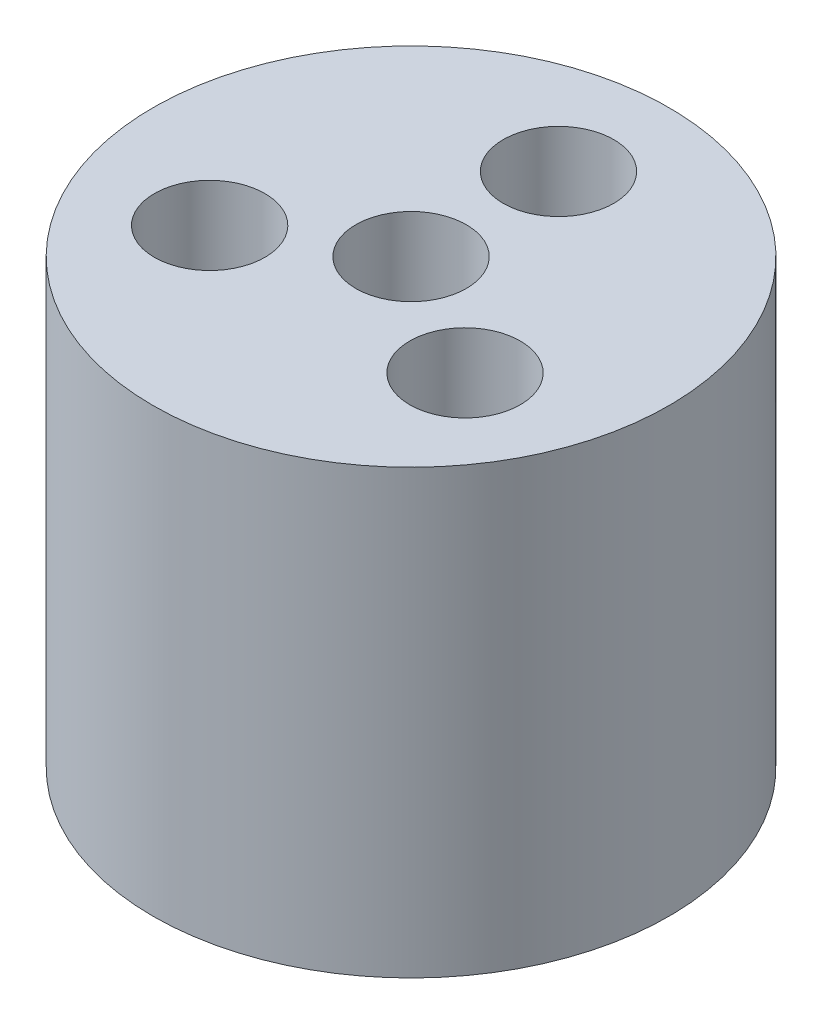
ISO-10303-21;
HEADER;
FILE_DESCRIPTION(('STEP AP214'),'2;1');
FILE_NAME('part.step','',(''),(''),'','','');
FILE_SCHEMA(('AUTOMOTIVE_DESIGN { 1 0 10303 214 1 1 1 1 }'));
ENDSEC;
DATA;
#1=APPLICATION_CONTEXT('core data for automotive mechanical design processes');
#2=APPLICATION_PROTOCOL_DEFINITION('international standard','automotive_design',2000,#1);
#3=PRODUCT_CONTEXT('',#1,'mechanical');
#4=PRODUCT('Part','Part','',(#3));
#5=PRODUCT_RELATED_PRODUCT_CATEGORY('part','',(#4));
#6=PRODUCT_DEFINITION_FORMATION('','',#4);
#7=PRODUCT_DEFINITION_CONTEXT('part definition',#1,'design');
#8=PRODUCT_DEFINITION('design','',#6,#7);
#9=PRODUCT_DEFINITION_SHAPE('','',#8);
#10=(LENGTH_UNIT() NAMED_UNIT(*) SI_UNIT(.MILLI.,.METRE.));
#11=(NAMED_UNIT(*) PLANE_ANGLE_UNIT() SI_UNIT($,.RADIAN.));
#12=(NAMED_UNIT(*) SI_UNIT($,.STERADIAN.) SOLID_ANGLE_UNIT());
#13=UNCERTAINTY_MEASURE_WITH_UNIT(LENGTH_MEASURE(1.E-05),#10,'distance_accuracy_value','');
#14=(GEOMETRIC_REPRESENTATION_CONTEXT(3) GLOBAL_UNCERTAINTY_ASSIGNED_CONTEXT((#13)) GLOBAL_UNIT_ASSIGNED_CONTEXT((#10,
#11,#12)) REPRESENTATION_CONTEXT('',''));
#15=CARTESIAN_POINT('',(0.,0.,0.));
#16=DIRECTION('',(0.,0.,1.));
#17=DIRECTION('',(1.,0.,0.));
#18=AXIS2_PLACEMENT_3D('',#15,#16,#17);
#19=CARTESIAN_POINT('',(0.,24.,0.));
#20=DIRECTION('',(0.,-1.,0.));
#21=DIRECTION('',(0.,0.,-1.));
#22=AXIS2_PLACEMENT_3D('',#19,#20,#21);
#23=CYLINDRICAL_SURFACE('',#22,14.);
#24=CARTESIAN_POINT('',(0.,24.,0.));
#25=DIRECTION('',(0.,1.,0.));
#26=DIRECTION('',(0.,0.,1.));
#27=AXIS2_PLACEMENT_3D('',#24,#25,#26);
#28=CIRCLE('',#27,14.);
#29=CARTESIAN_POINT('',(0.,24.,14.));
#30=VERTEX_POINT('',#29);
#31=EDGE_CURVE('E10',#30,#30,#28,.T.);
#32=ORIENTED_EDGE('',*,*,#31,.F.);
#33=EDGE_LOOP('',(#32));
#34=FACE_BOUND('',#33,.T.);
#35=CARTESIAN_POINT('',(0.,0.,0.));
#36=DIRECTION('',(0.,1.,0.));
#37=DIRECTION('',(0.,0.,1.));
#38=AXIS2_PLACEMENT_3D('',#35,#36,#37);
#39=CIRCLE('',#38,14.);
#40=CARTESIAN_POINT('',(0.,0.,14.));
#41=VERTEX_POINT('',#40);
#42=EDGE_CURVE('E42',#41,#41,#39,.T.);
#43=ORIENTED_EDGE('',*,*,#42,.T.);
#44=EDGE_LOOP('',(#43));
#45=FACE_BOUND('',#44,.T.);
#46=ADVANCED_FACE('F40',(#34,#45),#23,.T.);
#47=CARTESIAN_POINT('',(0.,24.,0.));
#48=DIRECTION('',(0.,1.,0.));
#49=DIRECTION('',(0.,0.,1.));
#50=AXIS2_PLACEMENT_3D('',#47,#48,#49);
#51=PLANE('',#50);
#52=CARTESIAN_POINT('',(0.,24.,0.));
#53=DIRECTION('',(0.,1.,0.));
#54=DIRECTION('',(0.,0.,1.));
#55=AXIS2_PLACEMENT_3D('',#52,#53,#54);
#56=CIRCLE('',#55,3.);
#57=CARTESIAN_POINT('',(0.,24.,3.));
#58=VERTEX_POINT('',#57);
#59=EDGE_CURVE('E102',#58,#58,#56,.T.);
#60=ORIENTED_EDGE('',*,*,#59,.F.);
#61=EDGE_LOOP('',(#60));
#62=FACE_BOUND('',#61,.T.);
#63=CARTESIAN_POINT('',(6.92820323027602,24.,3.9999999999997));
#64=DIRECTION('',(0.,1.,0.));
#65=DIRECTION('',(0.,0.,1.));
#66=AXIS2_PLACEMENT_3D('',#63,#64,#65);
#67=CIRCLE('',#66,3.00000000000044);
#68=CARTESIAN_POINT('',(6.92820323027602,24.,7.00000000000014));
#69=VERTEX_POINT('',#68);
#70=EDGE_CURVE('E56',#69,#69,#67,.T.);
#71=ORIENTED_EDGE('',*,*,#70,.F.);
#72=EDGE_LOOP('',(#71));
#73=FACE_BOUND('',#72,.T.);
#74=CARTESIAN_POINT('',(0.,24.,-8.));
#75=DIRECTION('',(0.,1.,0.));
#76=DIRECTION('',(0.,0.,1.));
#77=AXIS2_PLACEMENT_3D('',#74,#75,#76);
#78=CIRCLE('',#77,3.);
#79=CARTESIAN_POINT('',(0.,24.,-5.));
#80=VERTEX_POINT('',#79);
#81=EDGE_CURVE('E106',#80,#80,#78,.T.);
#82=ORIENTED_EDGE('',*,*,#81,.F.);
#83=EDGE_LOOP('',(#82));
#84=FACE_BOUND('',#83,.T.);
#85=CARTESIAN_POINT('',(-6.928203230275,24.,4.0000000000003));
#86=DIRECTION('',(0.,1.,0.));
#87=DIRECTION('',(0.,0.,1.));
#88=AXIS2_PLACEMENT_3D('',#85,#86,#87);
#89=CIRCLE('',#88,3.00000000000065);
#90=CARTESIAN_POINT('',(-6.928203230275,24.,7.00000000000095));
#91=VERTEX_POINT('',#90);
#92=EDGE_CURVE('E55',#91,#91,#89,.T.);
#93=ORIENTED_EDGE('',*,*,#92,.F.);
#94=EDGE_LOOP('',(#93));
#95=FACE_BOUND('',#94,.T.);
#96=ORIENTED_EDGE('',*,*,#31,.T.);
#97=EDGE_LOOP('',(#96));
#98=FACE_BOUND('',#97,.T.);
#99=ADVANCED_FACE('F84',(#62,#73,#84,#95,#98),#51,.T.);
#100=CARTESIAN_POINT('',(0.,0.,0.));
#101=DIRECTION('',(0.,1.,0.));
#102=DIRECTION('',(0.,0.,1.));
#103=AXIS2_PLACEMENT_3D('',#100,#101,#102);
#104=PLANE('',#103);
#105=CARTESIAN_POINT('',(0.,0.,0.));
#106=DIRECTION('',(0.,1.,0.));
#107=DIRECTION('',(0.,0.,1.));
#108=AXIS2_PLACEMENT_3D('',#105,#106,#107);
#109=CIRCLE('',#108,3.);
#110=CARTESIAN_POINT('',(0.,0.,3.));
#111=VERTEX_POINT('',#110);
#112=EDGE_CURVE('E37',#111,#111,#109,.T.);
#113=ORIENTED_EDGE('',*,*,#112,.T.);
#114=EDGE_LOOP('',(#113));
#115=FACE_BOUND('',#114,.T.);
#116=CARTESIAN_POINT('',(6.92820323027602,0.,3.9999999999997));
#117=DIRECTION('',(0.,1.,0.));
#118=DIRECTION('',(0.,0.,1.));
#119=AXIS2_PLACEMENT_3D('',#116,#117,#118);
#120=CIRCLE('',#119,3.00000000000044);
#121=CARTESIAN_POINT('',(6.92820323027602,0.,7.00000000000014));
#122=VERTEX_POINT('',#121);
#123=EDGE_CURVE('E47',#122,#122,#120,.T.);
#124=ORIENTED_EDGE('',*,*,#123,.T.);
#125=EDGE_LOOP('',(#124));
#126=FACE_BOUND('',#125,.T.);
#127=CARTESIAN_POINT('',(0.,0.,-8.));
#128=DIRECTION('',(0.,1.,0.));
#129=DIRECTION('',(0.,0.,1.));
#130=AXIS2_PLACEMENT_3D('',#127,#128,#129);
#131=CIRCLE('',#130,3.);
#132=CARTESIAN_POINT('',(0.,0.,-5.));
#133=VERTEX_POINT('',#132);
#134=EDGE_CURVE('E59',#133,#133,#131,.T.);
#135=ORIENTED_EDGE('',*,*,#134,.T.);
#136=EDGE_LOOP('',(#135));
#137=FACE_BOUND('',#136,.T.);
#138=CARTESIAN_POINT('',(-6.928203230275,0.,4.0000000000003));
#139=DIRECTION('',(0.,1.,0.));
#140=DIRECTION('',(0.,0.,1.));
#141=AXIS2_PLACEMENT_3D('',#138,#139,#140);
#142=CIRCLE('',#141,3.00000000000065);
#143=CARTESIAN_POINT('',(-6.928203230275,0.,7.00000000000095));
#144=VERTEX_POINT('',#143);
#145=EDGE_CURVE('E54',#144,#144,#142,.T.);
#146=ORIENTED_EDGE('',*,*,#145,.T.);
#147=EDGE_LOOP('',(#146));
#148=FACE_BOUND('',#147,.T.);
#149=ORIENTED_EDGE('',*,*,#42,.F.);
#150=EDGE_LOOP('',(#149));
#151=FACE_BOUND('',#150,.T.);
#152=ADVANCED_FACE('F63',(#115,#126,#137,#148,#151),#104,.F.);
#153=CARTESIAN_POINT('',(-6.928203230275,-5.,4.0000000000003));
#154=DIRECTION('',(0.,1.,0.));
#155=DIRECTION('',(0.,0.,1.));
#156=AXIS2_PLACEMENT_3D('',#153,#154,#155);
#157=CYLINDRICAL_SURFACE('',#156,3.00000000000065);
#158=CARTESIAN_POINT('',(-6.928203230275,24.,7.00000000000095));
#159=CARTESIAN_POINT('',(-6.928203230275,23.75,7.00000000000095));
#160=CARTESIAN_POINT('',(-6.928203230275,23.5,7.00000000000095));
#161=CARTESIAN_POINT('',(-6.928203230275,23.,7.00000000000095));
#162=CARTESIAN_POINT('',(-6.928203230275,22.75,7.00000000000095));
#163=CARTESIAN_POINT('',(-6.928203230275,22.25,7.00000000000095));
#164=CARTESIAN_POINT('',(-6.928203230275,22.,7.00000000000095));
#165=CARTESIAN_POINT('',(-6.928203230275,21.5,7.00000000000095));
#166=CARTESIAN_POINT('',(-6.928203230275,21.25,7.00000000000095));
#167=CARTESIAN_POINT('',(-6.928203230275,20.75,7.00000000000095));
#168=CARTESIAN_POINT('',(-6.928203230275,20.5,7.00000000000095));
#169=CARTESIAN_POINT('',(-6.928203230275,20.,7.00000000000095));
#170=CARTESIAN_POINT('',(-6.928203230275,19.75,7.00000000000095));
#171=CARTESIAN_POINT('',(-6.928203230275,19.25,7.00000000000095));
#172=CARTESIAN_POINT('',(-6.928203230275,19.,7.00000000000095));
#173=CARTESIAN_POINT('',(-6.928203230275,18.5,7.00000000000095));
#174=CARTESIAN_POINT('',(-6.928203230275,18.25,7.00000000000095));
#175=CARTESIAN_POINT('',(-6.928203230275,17.75,7.00000000000095));
#176=CARTESIAN_POINT('',(-6.928203230275,17.5,7.00000000000095));
#177=CARTESIAN_POINT('',(-6.928203230275,17.,7.00000000000095));
#178=CARTESIAN_POINT('',(-6.928203230275,16.75,7.00000000000095));
#179=CARTESIAN_POINT('',(-6.928203230275,16.25,7.00000000000095));
#180=CARTESIAN_POINT('',(-6.928203230275,16.,7.00000000000095));
#181=CARTESIAN_POINT('',(-6.928203230275,15.5,7.00000000000095));
#182=CARTESIAN_POINT('',(-6.928203230275,15.25,7.00000000000095));
#183=CARTESIAN_POINT('',(-6.928203230275,14.75,7.00000000000095));
#184=CARTESIAN_POINT('',(-6.928203230275,14.5,7.00000000000095));
#185=CARTESIAN_POINT('',(-6.928203230275,14.,7.00000000000095));
#186=CARTESIAN_POINT('',(-6.928203230275,13.75,7.00000000000095));
#187=CARTESIAN_POINT('',(-6.928203230275,13.25,7.00000000000095));
#188=CARTESIAN_POINT('',(-6.928203230275,13.,7.00000000000095));
#189=CARTESIAN_POINT('',(-6.928203230275,12.5,7.00000000000095));
#190=CARTESIAN_POINT('',(-6.928203230275,12.25,7.00000000000095));
#191=CARTESIAN_POINT('',(-6.928203230275,11.75,7.00000000000095));
#192=CARTESIAN_POINT('',(-6.928203230275,11.5,7.00000000000095));
#193=CARTESIAN_POINT('',(-6.928203230275,11.,7.00000000000095));
#194=CARTESIAN_POINT('',(-6.928203230275,10.75,7.00000000000095));
#195=CARTESIAN_POINT('',(-6.928203230275,10.25,7.00000000000095));
#196=CARTESIAN_POINT('',(-6.928203230275,10.,7.00000000000095));
#197=CARTESIAN_POINT('',(-6.928203230275,9.5,7.00000000000095));
#198=CARTESIAN_POINT('',(-6.928203230275,9.25,7.00000000000095));
#199=CARTESIAN_POINT('',(-6.928203230275,8.75,7.00000000000095));
#200=CARTESIAN_POINT('',(-6.928203230275,8.5,7.00000000000095));
#201=CARTESIAN_POINT('',(-6.928203230275,8.,7.00000000000095));
#202=CARTESIAN_POINT('',(-6.928203230275,7.75,7.00000000000095));
#203=CARTESIAN_POINT('',(-6.928203230275,7.25,7.00000000000095));
#204=CARTESIAN_POINT('',(-6.928203230275,7.,7.00000000000095));
#205=CARTESIAN_POINT('',(-6.928203230275,6.5,7.00000000000095));
#206=CARTESIAN_POINT('',(-6.928203230275,6.25,7.00000000000095));
#207=CARTESIAN_POINT('',(-6.928203230275,5.75,7.00000000000095));
#208=CARTESIAN_POINT('',(-6.928203230275,5.5,7.00000000000095));
#209=CARTESIAN_POINT('',(-6.928203230275,5.,7.00000000000095));
#210=CARTESIAN_POINT('',(-6.928203230275,4.75,7.00000000000095));
#211=CARTESIAN_POINT('',(-6.928203230275,4.25,7.00000000000095));
#212=CARTESIAN_POINT('',(-6.928203230275,4.,7.00000000000095));
#213=CARTESIAN_POINT('',(-6.928203230275,3.5,7.00000000000095));
#214=CARTESIAN_POINT('',(-6.928203230275,3.25,7.00000000000095));
#215=CARTESIAN_POINT('',(-6.928203230275,2.75,7.00000000000095));
#216=CARTESIAN_POINT('',(-6.928203230275,2.5,7.00000000000095));
#217=CARTESIAN_POINT('',(-6.928203230275,2.,7.00000000000095));
#218=CARTESIAN_POINT('',(-6.928203230275,1.75,7.00000000000095));
#219=CARTESIAN_POINT('',(-6.928203230275,1.25,7.00000000000095));
#220=CARTESIAN_POINT('',(-6.928203230275,1.,7.00000000000095));
#221=CARTESIAN_POINT('',(-6.928203230275,0.5,7.00000000000095));
#222=CARTESIAN_POINT('',(-6.928203230275,0.25,7.00000000000095));
#223=CARTESIAN_POINT('',(-6.928203230275,0.,7.00000000000095));
#224=B_SPLINE_CURVE_WITH_KNOTS('',3,(#158,#159,#160,#161,#162,#163,#164,#165,#166,#167,#168,
#169,#170,#171,#172,#173,#174,#175,#176,#177,#178,#179,#180,#181,#182,#183,#184,#185,#186,#187,
#188,#189,#190,#191,#192,#193,#194,#195,#196,#197,#198,#199,#200,#201,#202,#203,#204,#205,#206,
#207,#208,#209,#210,#211,#212,#213,#214,#215,#216,#217,#218,#219,#220,#221,#222,#223),
.UNSPECIFIED.,.F.,.F.,(4,2,2,2,2,2,2,2,2,2,2,2,2,2,2,2,2,2,2,2,2,2,2,2,2,2,2,2,2,2,2,2,4),(0.,
0.750000000000001,1.5,2.25,3.,3.75,4.5,5.25,6.,6.75,7.5,8.25,9.,9.75,10.5,11.25,12.,12.75,13.5,
14.25,15.,15.75,16.5,17.25,18.,18.75,19.5,20.25,21.,21.75,22.5,23.25,24.),.UNSPECIFIED.);
#225=EDGE_CURVE('BSEAM77',#91,#144,#224,.T.);
#226=ORIENTED_EDGE('',*,*,#92,.T.);
#227=ORIENTED_EDGE('',*,*,#145,.F.);
#228=ORIENTED_EDGE('',*,*,#225,.T.);
#229=ORIENTED_EDGE('',*,*,#225,.F.);
#230=EDGE_LOOP('',(#226,#228,#227,#229));
#231=FACE_BOUND('',#230,.T.);
#232=ADVANCED_FACE('F77',(#231),#157,.F.);
#233=CARTESIAN_POINT('',(0.,-5.,-8.));
#234=DIRECTION('',(0.,1.,0.));
#235=DIRECTION('',(0.,0.,1.));
#236=AXIS2_PLACEMENT_3D('',#233,#234,#235);
#237=CYLINDRICAL_SURFACE('',#236,3.);
#238=CARTESIAN_POINT('',(0.,24.,-5.));
#239=CARTESIAN_POINT('',(0.,23.75,-5.));
#240=CARTESIAN_POINT('',(0.,23.5,-5.));
#241=CARTESIAN_POINT('',(0.,23.,-5.));
#242=CARTESIAN_POINT('',(0.,22.75,-5.));
#243=CARTESIAN_POINT('',(0.,22.25,-5.));
#244=CARTESIAN_POINT('',(0.,22.,-5.));
#245=CARTESIAN_POINT('',(0.,21.5,-5.));
#246=CARTESIAN_POINT('',(0.,21.25,-5.));
#247=CARTESIAN_POINT('',(0.,20.75,-5.));
#248=CARTESIAN_POINT('',(0.,20.5,-5.));
#249=CARTESIAN_POINT('',(0.,20.,-5.));
#250=CARTESIAN_POINT('',(0.,19.75,-5.));
#251=CARTESIAN_POINT('',(0.,19.25,-5.));
#252=CARTESIAN_POINT('',(0.,19.,-5.));
#253=CARTESIAN_POINT('',(0.,18.5,-5.));
#254=CARTESIAN_POINT('',(0.,18.25,-5.));
#255=CARTESIAN_POINT('',(0.,17.75,-5.));
#256=CARTESIAN_POINT('',(0.,17.5,-5.));
#257=CARTESIAN_POINT('',(0.,17.,-5.));
#258=CARTESIAN_POINT('',(0.,16.75,-5.));
#259=CARTESIAN_POINT('',(0.,16.25,-5.));
#260=CARTESIAN_POINT('',(0.,16.,-5.));
#261=CARTESIAN_POINT('',(0.,15.5,-5.));
#262=CARTESIAN_POINT('',(0.,15.25,-5.));
#263=CARTESIAN_POINT('',(0.,14.75,-5.));
#264=CARTESIAN_POINT('',(0.,14.5,-5.));
#265=CARTESIAN_POINT('',(0.,14.,-5.));
#266=CARTESIAN_POINT('',(0.,13.75,-5.));
#267=CARTESIAN_POINT('',(0.,13.25,-5.));
#268=CARTESIAN_POINT('',(0.,13.,-5.));
#269=CARTESIAN_POINT('',(0.,12.5,-5.));
#270=CARTESIAN_POINT('',(0.,12.25,-5.));
#271=CARTESIAN_POINT('',(0.,11.75,-5.));
#272=CARTESIAN_POINT('',(0.,11.5,-5.));
#273=CARTESIAN_POINT('',(0.,11.,-5.));
#274=CARTESIAN_POINT('',(0.,10.75,-5.));
#275=CARTESIAN_POINT('',(0.,10.25,-5.));
#276=CARTESIAN_POINT('',(0.,10.,-5.));
#277=CARTESIAN_POINT('',(0.,9.5,-5.));
#278=CARTESIAN_POINT('',(0.,9.25,-5.));
#279=CARTESIAN_POINT('',(0.,8.75,-5.));
#280=CARTESIAN_POINT('',(0.,8.5,-5.));
#281=CARTESIAN_POINT('',(0.,8.,-5.));
#282=CARTESIAN_POINT('',(0.,7.75,-5.));
#283=CARTESIAN_POINT('',(0.,7.25,-5.));
#284=CARTESIAN_POINT('',(0.,7.,-5.));
#285=CARTESIAN_POINT('',(0.,6.5,-5.));
#286=CARTESIAN_POINT('',(0.,6.25,-5.));
#287=CARTESIAN_POINT('',(0.,5.75,-5.));
#288=CARTESIAN_POINT('',(0.,5.5,-5.));
#289=CARTESIAN_POINT('',(0.,5.,-5.));
#290=CARTESIAN_POINT('',(0.,4.75,-5.));
#291=CARTESIAN_POINT('',(0.,4.25,-5.));
#292=CARTESIAN_POINT('',(0.,4.,-5.));
#293=CARTESIAN_POINT('',(0.,3.5,-5.));
#294=CARTESIAN_POINT('',(0.,3.25,-5.));
#295=CARTESIAN_POINT('',(0.,2.75,-5.));
#296=CARTESIAN_POINT('',(0.,2.5,-5.));
#297=CARTESIAN_POINT('',(0.,2.,-5.));
#298=CARTESIAN_POINT('',(0.,1.75,-5.));
#299=CARTESIAN_POINT('',(0.,1.25,-5.));
#300=CARTESIAN_POINT('',(0.,1.,-5.));
#301=CARTESIAN_POINT('',(0.,0.5,-5.));
#302=CARTESIAN_POINT('',(0.,0.25,-5.));
#303=CARTESIAN_POINT('',(0.,0.,-5.));
#304=B_SPLINE_CURVE_WITH_KNOTS('',3,(#238,#239,#240,#241,#242,#243,#244,#245,#246,#247,#248,
#249,#250,#251,#252,#253,#254,#255,#256,#257,#258,#259,#260,#261,#262,#263,#264,#265,#266,#267,
#268,#269,#270,#271,#272,#273,#274,#275,#276,#277,#278,#279,#280,#281,#282,#283,#284,#285,#286,
#287,#288,#289,#290,#291,#292,#293,#294,#295,#296,#297,#298,#299,#300,#301,#302,#303),
.UNSPECIFIED.,.F.,.F.,(4,2,2,2,2,2,2,2,2,2,2,2,2,2,2,2,2,2,2,2,2,2,2,2,2,2,2,2,2,2,2,2,4),(0.,
0.750000000000001,1.5,2.25,3.,3.75,4.5,5.25,6.,6.75,7.5,8.25,9.,9.75,10.5,11.25,12.,12.75,13.5,
14.25,15.,15.75,16.5,17.25,18.,18.75,19.5,20.25,21.,21.75,22.5,23.25,24.),.UNSPECIFIED.);
#305=EDGE_CURVE('BSEAM69',#80,#133,#304,.T.);
#306=ORIENTED_EDGE('',*,*,#81,.T.);
#307=ORIENTED_EDGE('',*,*,#134,.F.);
#308=ORIENTED_EDGE('',*,*,#305,.T.);
#309=ORIENTED_EDGE('',*,*,#305,.F.);
#310=EDGE_LOOP('',(#306,#308,#307,#309));
#311=FACE_BOUND('',#310,.T.);
#312=ADVANCED_FACE('F69',(#311),#237,.F.);
#313=CARTESIAN_POINT('',(6.92820323027602,-5.,3.9999999999997));
#314=DIRECTION('',(0.,1.,0.));
#315=DIRECTION('',(0.,0.,1.));
#316=AXIS2_PLACEMENT_3D('',#313,#314,#315);
#317=CYLINDRICAL_SURFACE('',#316,3.00000000000044);
#318=CARTESIAN_POINT('',(6.92820323027602,24.,7.00000000000014));
#319=CARTESIAN_POINT('',(6.92820323027602,23.75,7.00000000000014));
#320=CARTESIAN_POINT('',(6.92820323027602,23.5,7.00000000000014));
#321=CARTESIAN_POINT('',(6.92820323027602,23.,7.00000000000014));
#322=CARTESIAN_POINT('',(6.92820323027602,22.75,7.00000000000014));
#323=CARTESIAN_POINT('',(6.92820323027602,22.25,7.00000000000014));
#324=CARTESIAN_POINT('',(6.92820323027602,22.,7.00000000000014));
#325=CARTESIAN_POINT('',(6.92820323027602,21.5,7.00000000000014));
#326=CARTESIAN_POINT('',(6.92820323027602,21.25,7.00000000000014));
#327=CARTESIAN_POINT('',(6.92820323027602,20.75,7.00000000000014));
#328=CARTESIAN_POINT('',(6.92820323027602,20.5,7.00000000000014));
#329=CARTESIAN_POINT('',(6.92820323027602,20.,7.00000000000014));
#330=CARTESIAN_POINT('',(6.92820323027602,19.75,7.00000000000014));
#331=CARTESIAN_POINT('',(6.92820323027602,19.25,7.00000000000014));
#332=CARTESIAN_POINT('',(6.92820323027602,19.,7.00000000000014));
#333=CARTESIAN_POINT('',(6.92820323027602,18.5,7.00000000000014));
#334=CARTESIAN_POINT('',(6.92820323027602,18.25,7.00000000000014));
#335=CARTESIAN_POINT('',(6.92820323027602,17.75,7.00000000000014));
#336=CARTESIAN_POINT('',(6.92820323027602,17.5,7.00000000000014));
#337=CARTESIAN_POINT('',(6.92820323027602,17.,7.00000000000014));
#338=CARTESIAN_POINT('',(6.92820323027602,16.75,7.00000000000014));
#339=CARTESIAN_POINT('',(6.92820323027602,16.25,7.00000000000014));
#340=CARTESIAN_POINT('',(6.92820323027602,16.,7.00000000000014));
#341=CARTESIAN_POINT('',(6.92820323027602,15.5,7.00000000000014));
#342=CARTESIAN_POINT('',(6.92820323027602,15.25,7.00000000000014));
#343=CARTESIAN_POINT('',(6.92820323027602,14.75,7.00000000000014));
#344=CARTESIAN_POINT('',(6.92820323027602,14.5,7.00000000000014));
#345=CARTESIAN_POINT('',(6.92820323027602,14.,7.00000000000014));
#346=CARTESIAN_POINT('',(6.92820323027602,13.75,7.00000000000014));
#347=CARTESIAN_POINT('',(6.92820323027602,13.25,7.00000000000014));
#348=CARTESIAN_POINT('',(6.92820323027602,13.,7.00000000000014));
#349=CARTESIAN_POINT('',(6.92820323027602,12.5,7.00000000000014));
#350=CARTESIAN_POINT('',(6.92820323027602,12.25,7.00000000000014));
#351=CARTESIAN_POINT('',(6.92820323027602,11.75,7.00000000000014));
#352=CARTESIAN_POINT('',(6.92820323027602,11.5,7.00000000000014));
#353=CARTESIAN_POINT('',(6.92820323027602,11.,7.00000000000014));
#354=CARTESIAN_POINT('',(6.92820323027602,10.75,7.00000000000014));
#355=CARTESIAN_POINT('',(6.92820323027602,10.25,7.00000000000014));
#356=CARTESIAN_POINT('',(6.92820323027602,10.,7.00000000000014));
#357=CARTESIAN_POINT('',(6.92820323027602,9.5,7.00000000000014));
#358=CARTESIAN_POINT('',(6.92820323027602,9.25,7.00000000000014));
#359=CARTESIAN_POINT('',(6.92820323027602,8.75,7.00000000000014));
#360=CARTESIAN_POINT('',(6.92820323027602,8.5,7.00000000000014));
#361=CARTESIAN_POINT('',(6.92820323027602,8.,7.00000000000014));
#362=CARTESIAN_POINT('',(6.92820323027602,7.75,7.00000000000014));
#363=CARTESIAN_POINT('',(6.92820323027602,7.25,7.00000000000014));
#364=CARTESIAN_POINT('',(6.92820323027602,7.,7.00000000000014));
#365=CARTESIAN_POINT('',(6.92820323027602,6.5,7.00000000000014));
#366=CARTESIAN_POINT('',(6.92820323027602,6.25,7.00000000000014));
#367=CARTESIAN_POINT('',(6.92820323027602,5.75,7.00000000000014));
#368=CARTESIAN_POINT('',(6.92820323027602,5.5,7.00000000000014));
#369=CARTESIAN_POINT('',(6.92820323027602,5.,7.00000000000014));
#370=CARTESIAN_POINT('',(6.92820323027602,4.75,7.00000000000014));
#371=CARTESIAN_POINT('',(6.92820323027602,4.25,7.00000000000014));
#372=CARTESIAN_POINT('',(6.92820323027602,4.,7.00000000000014));
#373=CARTESIAN_POINT('',(6.92820323027602,3.5,7.00000000000014));
#374=CARTESIAN_POINT('',(6.92820323027602,3.25,7.00000000000014));
#375=CARTESIAN_POINT('',(6.92820323027602,2.75,7.00000000000014));
#376=CARTESIAN_POINT('',(6.92820323027602,2.5,7.00000000000014));
#377=CARTESIAN_POINT('',(6.92820323027602,2.,7.00000000000014));
#378=CARTESIAN_POINT('',(6.92820323027602,1.75,7.00000000000014));
#379=CARTESIAN_POINT('',(6.92820323027602,1.25,7.00000000000014));
#380=CARTESIAN_POINT('',(6.92820323027602,1.,7.00000000000014));
#381=CARTESIAN_POINT('',(6.92820323027602,0.5,7.00000000000014));
#382=CARTESIAN_POINT('',(6.92820323027602,0.25,7.00000000000014));
#383=CARTESIAN_POINT('',(6.92820323027602,0.,7.00000000000014));
#384=B_SPLINE_CURVE_WITH_KNOTS('',3,(#318,#319,#320,#321,#322,#323,#324,#325,#326,#327,#328,
#329,#330,#331,#332,#333,#334,#335,#336,#337,#338,#339,#340,#341,#342,#343,#344,#345,#346,#347,
#348,#349,#350,#351,#352,#353,#354,#355,#356,#357,#358,#359,#360,#361,#362,#363,#364,#365,#366,
#367,#368,#369,#370,#371,#372,#373,#374,#375,#376,#377,#378,#379,#380,#381,#382,#383),
.UNSPECIFIED.,.F.,.F.,(4,2,2,2,2,2,2,2,2,2,2,2,2,2,2,2,2,2,2,2,2,2,2,2,2,2,2,2,2,2,2,2,4),(0.,
0.750000000000001,1.5,2.25,3.,3.75,4.5,5.25,6.,6.75,7.5,8.25,9.,9.75,10.5,11.25,12.,12.75,13.5,
14.25,15.,15.75,16.5,17.25,18.,18.75,19.5,20.25,21.,21.75,22.5,23.25,24.),.UNSPECIFIED.);
#385=EDGE_CURVE('BSEAM70',#69,#122,#384,.T.);
#386=ORIENTED_EDGE('',*,*,#70,.T.);
#387=ORIENTED_EDGE('',*,*,#123,.F.);
#388=ORIENTED_EDGE('',*,*,#385,.T.);
#389=ORIENTED_EDGE('',*,*,#385,.F.);
#390=EDGE_LOOP('',(#386,#388,#387,#389));
#391=FACE_BOUND('',#390,.T.);
#392=ADVANCED_FACE('F70',(#391),#317,.F.);
#393=CARTESIAN_POINT('',(0.,-5.,0.));
#394=DIRECTION('',(0.,1.,0.));
#395=DIRECTION('',(0.,0.,1.));
#396=AXIS2_PLACEMENT_3D('',#393,#394,#395);
#397=CYLINDRICAL_SURFACE('',#396,3.);
#398=CARTESIAN_POINT('',(0.,24.,3.));
#399=CARTESIAN_POINT('',(0.,23.75,3.));
#400=CARTESIAN_POINT('',(0.,23.5,3.));
#401=CARTESIAN_POINT('',(0.,23.,3.));
#402=CARTESIAN_POINT('',(0.,22.75,3.));
#403=CARTESIAN_POINT('',(0.,22.25,3.));
#404=CARTESIAN_POINT('',(0.,22.,3.));
#405=CARTESIAN_POINT('',(0.,21.5,3.));
#406=CARTESIAN_POINT('',(0.,21.25,3.));
#407=CARTESIAN_POINT('',(0.,20.75,3.));
#408=CARTESIAN_POINT('',(0.,20.5,3.));
#409=CARTESIAN_POINT('',(0.,20.,3.));
#410=CARTESIAN_POINT('',(0.,19.75,3.));
#411=CARTESIAN_POINT('',(0.,19.25,3.));
#412=CARTESIAN_POINT('',(0.,19.,3.));
#413=CARTESIAN_POINT('',(0.,18.5,3.));
#414=CARTESIAN_POINT('',(0.,18.25,3.));
#415=CARTESIAN_POINT('',(0.,17.75,3.));
#416=CARTESIAN_POINT('',(0.,17.5,3.));
#417=CARTESIAN_POINT('',(0.,17.,3.));
#418=CARTESIAN_POINT('',(0.,16.75,3.));
#419=CARTESIAN_POINT('',(0.,16.25,3.));
#420=CARTESIAN_POINT('',(0.,16.,3.));
#421=CARTESIAN_POINT('',(0.,15.5,3.));
#422=CARTESIAN_POINT('',(0.,15.25,3.));
#423=CARTESIAN_POINT('',(0.,14.75,3.));
#424=CARTESIAN_POINT('',(0.,14.5,3.));
#425=CARTESIAN_POINT('',(0.,14.,3.));
#426=CARTESIAN_POINT('',(0.,13.75,3.));
#427=CARTESIAN_POINT('',(0.,13.25,3.));
#428=CARTESIAN_POINT('',(0.,13.,3.));
#429=CARTESIAN_POINT('',(0.,12.5,3.));
#430=CARTESIAN_POINT('',(0.,12.25,3.));
#431=CARTESIAN_POINT('',(0.,11.75,3.));
#432=CARTESIAN_POINT('',(0.,11.5,3.));
#433=CARTESIAN_POINT('',(0.,11.,3.));
#434=CARTESIAN_POINT('',(0.,10.75,3.));
#435=CARTESIAN_POINT('',(0.,10.25,3.));
#436=CARTESIAN_POINT('',(0.,10.,3.));
#437=CARTESIAN_POINT('',(0.,9.5,3.));
#438=CARTESIAN_POINT('',(0.,9.25,3.));
#439=CARTESIAN_POINT('',(0.,8.75,3.));
#440=CARTESIAN_POINT('',(0.,8.5,3.));
#441=CARTESIAN_POINT('',(0.,8.,3.));
#442=CARTESIAN_POINT('',(0.,7.75,3.));
#443=CARTESIAN_POINT('',(0.,7.25,3.));
#444=CARTESIAN_POINT('',(0.,7.,3.));
#445=CARTESIAN_POINT('',(0.,6.5,3.));
#446=CARTESIAN_POINT('',(0.,6.25,3.));
#447=CARTESIAN_POINT('',(0.,5.75,3.));
#448=CARTESIAN_POINT('',(0.,5.5,3.));
#449=CARTESIAN_POINT('',(0.,5.,3.));
#450=CARTESIAN_POINT('',(0.,4.75,3.));
#451=CARTESIAN_POINT('',(0.,4.25,3.));
#452=CARTESIAN_POINT('',(0.,4.,3.));
#453=CARTESIAN_POINT('',(0.,3.5,3.));
#454=CARTESIAN_POINT('',(0.,3.25,3.));
#455=CARTESIAN_POINT('',(0.,2.75,3.));
#456=CARTESIAN_POINT('',(0.,2.5,3.));
#457=CARTESIAN_POINT('',(0.,2.,3.));
#458=CARTESIAN_POINT('',(0.,1.75,3.));
#459=CARTESIAN_POINT('',(0.,1.25,3.));
#460=CARTESIAN_POINT('',(0.,1.,3.));
#461=CARTESIAN_POINT('',(0.,0.5,3.));
#462=CARTESIAN_POINT('',(0.,0.25,3.));
#463=CARTESIAN_POINT('',(0.,0.,3.));
#464=B_SPLINE_CURVE_WITH_KNOTS('',3,(#398,#399,#400,#401,#402,#403,#404,#405,#406,#407,#408,
#409,#410,#411,#412,#413,#414,#415,#416,#417,#418,#419,#420,#421,#422,#423,#424,#425,#426,#427,
#428,#429,#430,#431,#432,#433,#434,#435,#436,#437,#438,#439,#440,#441,#442,#443,#444,#445,#446,
#447,#448,#449,#450,#451,#452,#453,#454,#455,#456,#457,#458,#459,#460,#461,#462,#463),
.UNSPECIFIED.,.F.,.F.,(4,2,2,2,2,2,2,2,2,2,2,2,2,2,2,2,2,2,2,2,2,2,2,2,2,2,2,2,2,2,2,2,4),(0.,
0.750000000000001,1.5,2.25,3.,3.75,4.5,5.25,6.,6.75,7.5,8.25,9.,9.75,10.5,11.25,12.,12.75,13.5,
14.25,15.,15.75,16.5,17.25,18.,18.75,19.5,20.25,21.,21.75,22.5,23.25,24.),.UNSPECIFIED.);
#465=EDGE_CURVE('BSEAM67',#58,#111,#464,.T.);
#466=ORIENTED_EDGE('',*,*,#59,.T.);
#467=ORIENTED_EDGE('',*,*,#112,.F.);
#468=ORIENTED_EDGE('',*,*,#465,.T.);
#469=ORIENTED_EDGE('',*,*,#465,.F.);
#470=EDGE_LOOP('',(#466,#468,#467,#469));
#471=FACE_BOUND('',#470,.T.);
#472=ADVANCED_FACE('F67',(#471),#397,.F.);
#473=CLOSED_SHELL('',(#46,#99,#152,#232,#312,#392,#472));
#474=MANIFOLD_SOLID_BREP('B2',#473);
#475=ADVANCED_BREP_SHAPE_REPRESENTATION('',(#18,#474),#14);
#476=SHAPE_DEFINITION_REPRESENTATION(#9,#475);
ENDSEC;
END-ISO-10303-21;
